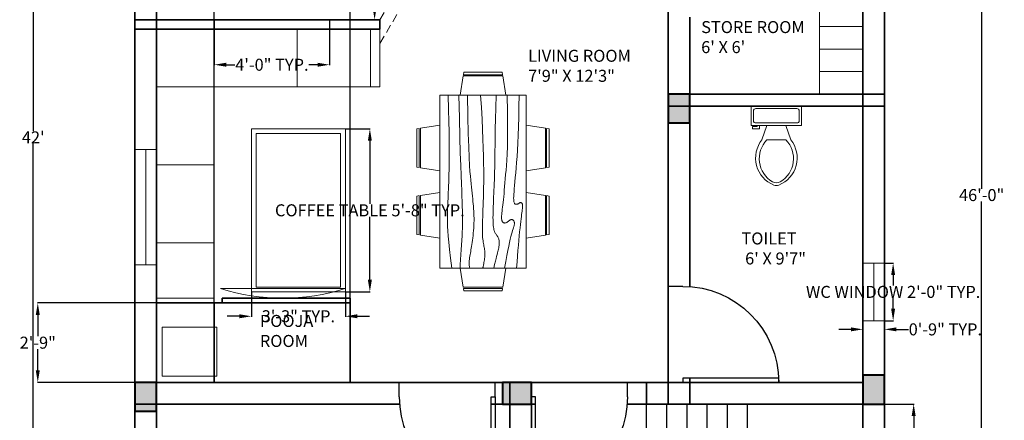
# Model space of a CAD drawing. Units: inches. Extents: x -54 to 881, y -122 to 681.
# Tile 5 of 6: x 472 to 881, y 254 to 421. Entities that reach past the tile are written whole.
import ezdxf

# ---------------------------------------------------------------- set-up
doc = ezdxf.new("R2010")
doc.units = ezdxf.units.IN
doc.header["$MEASUREMENT"] = 0
doc.linetypes.add('DASHED', pattern=[0.75, 0.5, -0.25])
for name, color, linetype, lineweight in [('A-ANNO-DIMS', 2, 'Continuous', 18), ('A-DOOR', 3, 'Continuous', 25), ('A-EQPM', 9, 'Continuous', 18), ('A-FLOR-CASE', 8, 'Continuous', 18), ('A-FLOR-FIXT', 9, 'Continuous', 18), ('A-FLOR-STRS', 7, 'Continuous', 25), ('A-FURN', 8, 'Continuous', 18), ('A-GLAZ', 4, 'Continuous', 20), ('A-WALL', 7, 'Continuous', 35), ('A-WALL-OVHD', 8, 'DASHED', 18)]:
    doc.layers.add(name, color=color, linetype=linetype, lineweight=lineweight)
doc.layers.add('A-AREA-IDEN', color=217, linetype='Continuous', lineweight=18, true_color=0x93278f)
doc.layers.add('A-COLS', color=240, linetype='Continuous', lineweight=40, true_color=0xed1f24)
doc.styles.get("Standard").update_dxf_attribs({"font": 'arial.ttf'})
doc.dimstyles.get("Standard").update_dxf_attribs({"dimtxt": 5, "dimasz": 5, "dimexe": 0.18, "dimexo": 0.0625, "dimgap": 0.09, "dimtad": 0, "dimtih": 1, "dimtoh": 1, "dimdec": 0, "dimzin": 0, "dimdsep": 46, "dimlunit": 3, "dimtxsty": 'Standard', "dimcen": 0.09, "dimadec": 0, "dimazin": 0, "dimtfac": 1, "dimtdec": 0, "dimtofl": 0, "dimtmove": 0, "dimatfit": 3, "dimfxl": 1, "dimtolj": 1, "dimtzin": 0, "dimarcsym": 0})

# ---------------------------------------------------------------- blocks, each defined once
blk = doc.blocks.new('*D14')
at = {"layer": 'A-ANNO-DIMS', "color": 0, "lineweight": -2, "transparency": 16777216}
for p, q in [((519.43, 624), (476.98, 624)), ((477.16, 619), (477.16, 374.6)), ((477.16, 125), (477.16, 369.4)), ((519.43, 120), (476.98, 120))]:
    blk.add_line(p, q, dxfattribs=at)
at = {"layer": 'A-ANNO-DIMS', "color": 0, "transparency": 16777216}
for points in [[(476.32, 619), (477.99, 619), (477.16, 624)], [(476.32, 125), (477.99, 125), (477.16, 120)]]:
    blk.add_solid(points, dxfattribs=at)
at = {"layer": 'Defpoints', "color": 0, "transparency": 16777216}
for p in [(519.49, 624), (477.16, 120), (519.49, 120)]:
    blk.add_point(p, dxfattribs=at)
at = {"layer": 'A-ANNO-DIMS', "color": 0, "transparency": 16777216, "insert": (477.16, 372), "char_height": 5, "attachment_point": 5}
blk.add_mtext("\\A1;42'", dxfattribs=at)
blk = doc.blocks.new('Toilet - top')
for p, q in [((9.5, -6), (9.5, -2)), ((-8, -8.5), (-8, -8)), ((-7, -8), (-7, -9.5)), ((-4, -8), (-6, -14)), ((4, -8), (6, -14)), ((-10, -8.5), (-8, -8.5)), ((-10, -9.5), (-10, -8.5)), ((-7, -9.5), (-10, -9.5)), ((4, -14), (-4, -14))]:
    blk.add_line(p, q)
blk.add_lwpolyline([(10.5, -8), (10.5, 0), (-10.5, 0), (-10.5, -8)], close=True)
for points in [[(-9.5, -2), (-9.5, -6)], [(8.5, -1), (-8.5, -1)], [(-8.5, -7), (8.5, -7)]]:
    blk.add_lwpolyline(points)
for centre, radius, start, end in [((-8.62, -1.88), 0.884, 81.8699, 188.1301), ((8.62, -1.88), 0.884, 351.8699, 98.1301), ((-8.62, -6.12), 0.884, 171.8699, 278.1301), ((8.62, -6.12), 0.884, 261.8699, 8.1301), ((3.52, -21.58), 12.17, 141.4691, 247.9714), ((4.2, -21.82), 11.33, 136.3677, 238.9468), ((-3.52, -21.58), 12.17, 292.0284, 38.5307), ((-4.2, -21.82), 11.33, 301.053, 43.6321), ((0, -27.88), 4, 245.7318, 294.2682), ((0, -29), 4, 254.8605, 285.1395)]:
    blk.add_arc(centre, radius, start, end)
blk = doc.blocks.new('Dining Set - 36 x 72 in.')
for p, q in [((-22.2343, 26.00059), (-23.4847, 17.99762)), ((-22.2304, 26), (-5.7608, 26)), ((-22, 27.5), (-22.1562, 26.50042)), ((-5.8416, 26.5), (-22.1534, 26.5)), ((-22, 27.5), (-6, 27.5)), ((-5.8437, 26.49966), (-6, 27.5)), ((-4.5152, 17.99762), (-5.7655, 25.99926)), ((5.7657, 26.00059), (4.5153, 17.99762)), ((5.7696, 26), (22.2392, 26)), ((6, 27.5), (5.8438, 26.50042)), ((22.1584, 26.5), (5.8466, 26.5)), ((6, 27.5), (22, 27.5)), ((22.1563, 26.49966), (22, 27.5)), ((23.4848, 17.99762), (22.2345, 25.99926)), ((36, 18), (-36, 18)), ((-36, 18), (-36, -18)), ((36, -18), (36, 18)), ((-44.0006, 8.23428), (-35.9976, 9.48474)), ((-44, 8.23041), (-44, -8.23915)), ((44.0006, 8.23428), (35.9976, 9.48474)), ((44, 8.23041), (44, -8.23915)), ((-45.5, 8), (-44.5004, 8.15617)), ((-45.5, 8), (-45.5, -8)), ((-44.5, -8.15843), (-44.5, 8.15338)), ((44.5, -8.15843), (44.5, 8.15338)), ((45.5, 8), (44.5005, 8.15617)), ((45.5, 8), (45.5, -8)), ((-44.4997, -8.15631), (-45.5, -8)), ((44.4997, -8.15631), (45.5, -8)), ((-35.9976, -9.48476), (-43.9993, -8.2345)), ((35.9976, -9.48476), (43.9993, -8.2345)), ((-36, -18), (36, -18)), ((-22.2343, -26.0006), (-23.4847, -17.99762)), ((-4.5152, -17.99762), (-5.7655, -25.99928)), ((5.7657, -26.0006), (4.5153, -17.99762)), ((23.4848, -17.99762), (22.2345, -25.99928)), ((-22.2304, -26), (-5.7608, -26)), ((-22, -27.5), (-22.1562, -26.50044)), ((-5.8416, -26.5), (-22.1534, -26.5)), ((-22, -27.5), (-6, -27.5)), ((-5.8437, -26.49967), (-6, -27.5)), ((5.7696, -26), (22.2392, -26)), ((6, -27.5), (5.8438, -26.50044)), ((22.1584, -26.5), (5.8466, -26.5)), ((6, -27.5), (22, -27.5)), ((22.1563, -26.49967), (22, -27.5))]:
    blk.add_line(p, q)
for points in [[(-36, 15), (-31.1772, 14.97754), (-26.8079, 14.91406), (-22.8538, 14.81543), (-19.276, 14.6875), (-16.0362, 14.53613), (-13.0957, 14.36718), (-10.4159, 14.18652), (-7.9583, 14), (-5.6904, 13.81315), (-3.6035, 13.63021), (-1.6954, 13.45508), (0.0365, 13.29166), (1.5945, 13.14388), (2.9811, 13.01562), (4.1988, 12.9108), (5.25, 12.83333), (6.1393, 12.78613), (6.8802, 12.76823), (7.4883, 12.77767), (7.9792, 12.8125), (8.3685, 12.87077), (8.6719, 12.95052), (8.9049, 13.0498), (9.0833, 13.16666), (9.2205, 13.29899), (9.3216, 13.44401), (9.3895, 13.59879), (9.4271, 13.76041), (9.4373, 13.92594), (9.4232, 14.09245), (9.3875, 14.257), (9.3333, 14.41666), (9.2638, 14.56917), (9.1836, 14.71484), (9.0975, 14.85465), (9.0104, 14.98958), (8.9272, 15.1206), (8.8529, 15.2487), (8.7922, 15.37483), (8.75, 15.5), (8.7305, 15.62467), (8.7344, 15.74739), (8.7617, 15.86621), (8.8125, 15.97916), (8.8867, 16.08431), (8.9844, 16.17968), (9.1055, 16.26334), (9.25, 16.33333), (9.4189, 16.38802), (9.6172, 16.42708), (9.8506, 16.45052), (10.125, 16.45833), (10.4463, 16.45052), (10.8203, 16.42708), (11.2529, 16.38802), (11.75, 16.33333), (12.3184, 16.26318), (12.9694, 16.17838), (13.7151, 16.07991), (14.5677, 15.96875), (15.5395, 15.84586), (16.6426, 15.71224), (17.8893, 15.56884), (19.2917, 15.41666), (20.859, 15.25667), (22.5879, 15.08984), (24.4721, 14.91715), (26.5052, 14.73958), (28.6809, 14.5581), (30.9929, 14.3737), (33.4347, 14.18733), (36, 14)], [(-36, 10), (-28.9766, 10.14274), (-23.1725, 10.20442), (-18.4241, 10.19775), (-14.5677, 10.13541), (-11.4399, 10.03011), (-8.877, 9.89453), (-6.7154, 9.74137), (-4.7917, 9.58333), (-2.9698, 9.43082), (-1.2246, 9.28515), (0.4415, 9.14534), (2.026, 9.01041), (3.5266, 8.87939), (4.9408, 8.7513), (6.266, 8.62516), (7.5, 8.5), (8.6411, 8.37549), (9.6914, 8.2539), (10.6538, 8.13818), (11.5312, 8.03125), (12.3267, 7.93603), (13.043, 7.85547), (13.6831, 7.79248), (14.25, 7.75), (14.7471, 7.7303), (15.1797, 7.73307), (15.5537, 7.75732), (15.875, 7.80208), (16.1494, 7.86637), (16.3828, 7.94922), (16.5811, 8.04964), (16.75, 8.16666), (16.8944, 8.29915), (17.0143, 8.44531), (17.1089, 8.60319), (17.1771, 8.77083), (17.218, 8.94629), (17.2305, 9.1276), (17.2137, 9.31282), (17.1667, 9.5), (17.0895, 9.6875), (16.987, 9.875), (16.8649, 10.0625), (16.7292, 10.25), (16.5856, 10.4375), (16.4401, 10.625), (16.2985, 10.8125), (16.1667, 11), (16.05, 11.18733), (15.9518, 11.3737), (15.8752, 11.5581), (15.8229, 11.73958), (15.798, 11.91715), (15.8034, 12.08984), (15.842, 12.25667), (15.9167, 12.41666), (16.0295, 12.56836), (16.1784, 12.70833), (16.3605, 12.83268), (16.5729, 12.9375), (16.8127, 13.01888), (17.0768, 13.07291), (17.3625, 13.0957), (17.6667, 13.08333), (17.9894, 13.03312), (18.3418, 12.94726), (18.7382, 12.82918), (19.1927, 12.68229), (19.7195, 12.51001), (20.3327, 12.31575), (21.0465, 12.10294), (21.875, 11.875), (22.8357, 11.63354), (23.959, 11.37304), (25.2786, 11.08618), (26.8282, 10.76562), (28.6414, 10.40405), (30.752, 9.99414), (33.1936, 9.52856), (36, 9)], [(-36, 5.5), (-30.7157, 5.3348), (-26.069, 5.20963), (-21.9946, 5.11767), (-18.4271, 5.05208), (-15.3009, 5.00602), (-12.5508, 4.97265), (-10.1112, 4.94515), (-7.9167, 4.91666), (-5.909, 4.88167), (-4.0586, 4.83984), (-2.3429, 4.79215), (-0.7396, 4.73958), (0.7739, 4.6831), (2.22, 4.6237), (3.6213, 4.56233), (5, 4.5), (6.373, 4.43782), (7.7344, 4.3776), (9.0723, 4.32129), (10.375, 4.27083), (11.6309, 4.22819), (12.8281, 4.19531), (13.9551, 4.17415), (15, 4.16666), (15.954, 4.17448), (16.819, 4.19791), (17.6001, 4.23698), (18.3021, 4.29166), (18.9299, 4.36198), (19.4883, 4.44791), (19.9823, 4.54948), (20.4167, 4.66666), (20.7969, 4.79899), (21.1302, 4.94401), (21.4245, 5.09879), (21.6875, 5.26041), (21.9271, 5.42594), (22.1511, 5.59245), (22.3672, 5.757), (22.5834, 5.91666), (22.8065, 6.06868), (23.0404, 6.21093), (23.2879, 6.34147), (23.5521, 6.45833), (23.8358, 6.55957), (24.142, 6.64323), (24.4735, 6.70735), (24.8334, 6.75), (25.2235, 6.76969), (25.642, 6.76692), (26.0858, 6.74267), (26.5521, 6.69791), (27.0379, 6.63362), (27.5404, 6.55078), (28.0565, 6.45036), (28.5834, 6.33333), (29.1242, 6.19987), (29.7071, 6.04687), (30.3661, 5.87044), (31.1354, 5.66666), (32.0493, 5.43164), (33.142, 5.16146), (34.4475, 4.85221), (36, 4.5)], [(-36, -1), (-30.7915, -0.6591), (-26.0195, -0.38216), (-21.6519, -0.16284), (-17.6563, 0.00521), (-14.0005, 0.12833), (-10.6523, 0.21289), (-7.5796, 0.26522), (-4.75, 0.29166), (-2.134, 0.29793), (0.2878, 0.28711), (2.5317, 0.26163), (4.6146, 0.22396), (6.5529, 0.17651), (8.3633, 0.12174), (10.0623, 0.06209), (11.6667, 0), (13.1899, -0.06201), (14.6341, -0.1211), (15.9982, -0.17432), (17.2813, -0.21875), (18.4823, -0.25147), (19.6003, -0.26953), (20.6343, -0.27002), (21.5834, -0.25), (22.4481, -0.20768), (23.2357, -0.14584), (23.9549, -0.06836), (24.6146, 0.02083), (25.2235, 0.11784), (25.7904, 0.21875), (26.3241, 0.31966), (26.8334, 0.41666), (27.3265, 0.50618), (27.8099, 0.58593), (28.2894, 0.65397), (28.7709, 0.70833), (29.2601, 0.74707), (29.763, 0.76823), (30.2855, 0.76985), (30.8334, 0.75), (31.4088, 0.70784), (31.9994, 0.64713), (32.589, 0.57275), (33.1615, 0.48958), (33.7008, 0.4025), (34.1908, 0.3164), (34.6153, 0.23616), (34.9584, 0.16666), (35.2099, 0.11165), (35.3848, 0.07031), (35.504, 0.04069), (35.5886, 0.02083), (35.6594, 0.00879), (35.7377, 0.0026), (35.8442, 0.00032), (36, 0)], [(-36, -6.5), (-27.1843, -6.31267), (-20.084, -6.1263), (-14.469, -5.9419), (-10.1094, -5.76042), (-6.7752, -5.58285), (-4.2363, -5.41016), (-2.2629, -5.24333), (-0.625, -5.08334), (0.8708, -4.93099), (2.2715, -4.78646), (3.5872, -4.64974), (4.8281, -4.52084), (6.0046, -4.39974), (7.127, -4.28646), (8.2053, -4.18099), (9.25, -4.08334), (10.2705, -3.99382), (11.2734, -3.91407), (12.2647, -3.84603), (13.25, -3.79167), (14.2354, -3.75293), (15.2266, -3.73177), (16.2295, -3.73015), (17.25, -3.75), (18.2912, -3.79248), (19.3451, -3.85547), (20.4009, -3.93604), (21.4479, -4.03125), (22.4754, -4.13819), (23.4727, -4.25391), (24.4289, -4.37549), (25.3334, -4.5), (26.1785, -4.62492), (26.9694, -4.74935), (27.7145, -4.87281), (28.4219, -4.99479), (29.1, -5.11483), (29.7572, -5.23242), (30.4016, -5.34709), (31.0417, -5.45834), (31.6837, -5.56437), (32.3262, -5.65821), (32.9658, -5.73153), (33.599, -5.77604), (34.2224, -5.78345), (34.8327, -5.74545), (35.4264, -5.65373), (36, -5.5)], [(-36, -10), (-26.4022, -9.81299), (-18.4675, -9.62891), (-11.9839, -9.45069), (-6.7396, -9.28125), (-2.5226, -9.12354), (0.8789, -8.98047), (3.6769, -8.85498), (6.0833, -8.75), (8.2767, -8.66765), (10.3021, -8.60677), (12.1712, -8.56543), (13.8958, -8.54167), (15.4876, -8.53353), (16.9583, -8.53907), (18.3197, -8.55632), (19.5834, -8.58334), (20.7616, -8.61841), (21.8685, -8.66081), (22.9188, -8.71004), (23.9271, -8.76563), (24.9081, -8.82707), (25.8763, -8.89388), (26.8465, -8.96558), (27.8334, -9.04167), (28.8474, -9.12118), (29.8828, -9.20117), (30.93, -9.27824), (31.9792, -9.34896), (33.0205, -9.40991), (34.0443, -9.45768), (35.0407, -9.48885), (36, -9.5)], [(-36, -14.5), (-30.0881, -14.33513), (-25.0332, -14.21224), (-20.7312, -14.12647), (-17.0781, -14.07292), (-13.97, -14.04671), (-11.3027, -14.04297), (-8.9724, -14.05681), (-6.875, -14.08334), (-4.9224, -14.11833), (-3.0905, -14.16016), (-1.3709, -14.20785), (0.2448, -14.26042), (1.7647, -14.3169), (3.1973, -14.3763), (4.5507, -14.43767), (5.8333, -14.5), (7.0554, -14.5621), (8.235, -14.62175), (9.3922, -14.67652), (10.5469, -14.72396), (11.7192, -14.76164), (12.929, -14.78711), (14.1965, -14.79794), (15.5417, -14.79167), (16.9933, -14.76424), (18.6152, -14.70508), (20.4804, -14.60197), (22.6615, -14.44271), (25.2312, -14.21509), (28.2624, -13.9069), (31.8277, -13.50594), (36, -13)]]:
    blk.add_lwpolyline(points)
blk = doc.blocks.new('*U12')
for p, q in [((0, 0), (0, -6)), ((40, 0), (40, -6))]:
    blk.add_line(p, q)
blk.add_lwpolyline([(0, 0), (0, 40), (1.75, 40), (1.75, 0)], close=True)
blk.add_arc((0, 0), 40, 0, 90)
blk = doc.blocks.new('WIN-48X9')
for p, q in [((0, 0), (0, 9)), ((48, 0), (48, 9)), ((0, 4.5), (48, 4.5))]:
    blk.add_line(p, q)
blk = doc.blocks.new('WIN-24X9')
for p, q in [((0, 24), (9, 24)), ((4.5, 24), (4.5, 0)), ((0, 0), (9, 0))]:
    blk.add_line(p, q)
blk = doc.blocks.new('TV-52-PLAN')
blk.add_line((0, 4), (52, 4))
blk.add_arc((26, 86.41), 86.41, 252.4883, 287.5117)
blk = doc.blocks.new('LIVING-COFFEE-TABLE')
for points in [[(0, 67.86), (39.15, 67.86), (39.15, 0), (0, 0)], [(2, 65.86), (37.15, 65.86), (37.15, 2), (2, 2)]]:
    blk.add_lwpolyline(points, close=True)
blk = doc.blocks.new('STAIR-RETURN-FLIGHT')
for p, q in [((48, 93), (48, 141)), ((56.4, 93), (56.4, 141)), ((64.8, 93), (64.8, 141)), ((73.2, 93), (73.2, 141)), ((81.6, 93), (81.6, 141)), ((90, 93), (90, 141)), ((48, 0), (48, 93)), ((48, 93), (90, 93)), ((48, 91), (90, 91)), ((50, 0), (50, 93)), ((88, 0), (88, 93)), ((90, 0), (90, 93)), ((90, 93), (138, 93)), ((90, 85), (138, 85)), ((90, 77), (138, 77)), ((90, 69), (138, 69)), ((90, 61), (138, 61)), ((0, 57), (48, 57)), ((90, 53), (138, 53)), ((0, 49), (48, 49)), ((0, 41), (48, 41)), ((90, 45), (138, 45)), ((90, 37), (138, 37)), ((0, 33), (48, 33)), ((90, 29), (138, 29)), ((0, 25), (48, 25)), ((90, 21), (138, 21)), ((0, 17), (48, 17)), ((90, 13), (138, 13)), ((0, 9), (48, 9)), ((48, 2), (90, 2)), ((48, 0), (90, 0))]:
    blk.add_line(p, q)
blk = doc.blocks.new('STORAGE-RACK-72X18')
for p, q in [((0, 0), (0, 72)), ((0, 65.625), (18, 65.625)), ((0, 56.25), (18, 56.25)), ((0, 46.875), (18, 46.875)), ((0, 37.5), (18, 37.5)), ((0, 28.125), (18, 28.125)), ((0, 18.75), (18, 18.75)), ((0, 9.375), (18, 9.375)), ((0, 0), (18, 0))]:
    blk.add_line(p, q)
blk = doc.blocks.new('COL-9X12')
h = blk.add_hatch(color=256)
h.dxf.hatch_style = 1
h.paths.add_polyline_path([(9, 12), (0, 12), (0, 0), (9, 0)])
blk.add_lwpolyline([(0, 0), (9, 0), (9, 12), (0, 12)], close=True)
blk = doc.blocks.new('LIVING-SIDE-TABLE')
blk.add_lwpolyline([(0, 20.5), (22.77, 20.5), (22.77, 0), (0, 0)], close=True)
blk = doc.blocks.new('*D44')
at = {"layer": 'A-ANNO-DIMS', "color": 0, "lineweight": -2, "transparency": 16777216}
for p, q in [((831.55, 319.69), (835.27, 319.69)), ((835.09, 314.69), (835.09, 310.36)), ((835.09, 300.69), (835.09, 305.01)), ((831.55, 295.69), (835.27, 295.69))]:
    blk.add_line(p, q, dxfattribs=at)
at = {"layer": 'A-ANNO-DIMS', "color": 0, "transparency": 16777216}
for points in [[(834.26, 314.69), (835.92, 314.69), (835.09, 319.69)], [(834.26, 300.69), (835.92, 300.69), (835.09, 295.69)]]:
    blk.add_solid(points, dxfattribs=at)
at = {"layer": 'Defpoints', "color": 0, "transparency": 16777216}
for p in [(831.49, 319.69), (835.09, 319.69), (831.49, 295.69)]:
    blk.add_point(p, dxfattribs=at)
at = {"layer": 'A-ANNO-DIMS', "color": 0, "transparency": 16777216, "insert": (835.09, 307.69), "char_height": 5, "attachment_point": 5}
blk.add_mtext('\\A1;WC WINDOW 2\'-0" TYP.', dxfattribs=at)
blk = doc.blocks.new('*D45')
at = {"layer": 'A-ANNO-DIMS', "color": 0, "lineweight": -2, "transparency": 16777216}
for p, q in [((822.49, 295.62), (822.49, 291.91)), ((831.49, 295.62), (831.49, 291.91)), ((817.49, 292.09), (812.49, 292.09)), ((836.49, 292.09), (841.49, 292.09))]:
    blk.add_line(p, q, dxfattribs=at)
at = {"layer": 'A-ANNO-DIMS', "color": 0, "transparency": 16777216}
for points in [[(817.49, 292.92), (817.49, 291.25), (822.49, 292.09)], [(836.49, 292.92), (836.49, 291.25), (831.49, 292.09)]]:
    blk.add_solid(points, dxfattribs=at)
at = {"layer": 'Defpoints', "color": 0, "transparency": 16777216}
for p in [(822.49, 295.69), (831.49, 295.69), (831.49, 292.09)]:
    blk.add_point(p, dxfattribs=at)
at = {"layer": 'A-ANNO-DIMS', "color": 0, "transparency": 16777216, "insert": (856.82, 292.09), "char_height": 5, "attachment_point": 5}
blk.add_mtext('\\A1;0\'-9" TYP.', dxfattribs=at)
blk = doc.blocks.new('*D62')
at = {"layer": 'A-ANNO-DIMS', "color": 0, "lineweight": -2, "transparency": 16777216}
for p, q in [((607.15, 375.58), (617.45, 375.58)), ((617.27, 370.58), (617.27, 344.32)), ((617.27, 312.72), (617.27, 338.97)), ((607.15, 307.72), (617.45, 307.72))]:
    blk.add_line(p, q, dxfattribs=at)
at = {"layer": 'A-ANNO-DIMS', "color": 0, "transparency": 16777216}
for points in [[(616.44, 370.58), (618.1, 370.58), (617.27, 375.58)], [(616.44, 312.72), (618.1, 312.72), (617.27, 307.72)]]:
    blk.add_solid(points, dxfattribs=at)
at = {"layer": 'Defpoints', "color": 0, "transparency": 16777216}
for p in [(607.09, 375.58), (617.27, 375.58), (607.09, 307.72)]:
    blk.add_point(p, dxfattribs=at)
at = {"layer": 'A-ANNO-DIMS', "color": 0, "transparency": 16777216, "insert": (617.27, 341.65), "char_height": 5, "attachment_point": 5}
blk.add_mtext('\\A1;COFFEE TABLE 5\'-8" TYP.', dxfattribs=at)
blk = doc.blocks.new('*D63')
at = {"layer": 'A-ANNO-DIMS', "color": 0, "lineweight": -2, "transparency": 16777216}
for p, q in [((567.94, 307.66), (567.94, 297.36)), ((607.09, 307.66), (607.09, 297.36)), ((562.94, 297.54), (557.94, 297.54)), ((612.09, 297.54), (617.09, 297.54))]:
    blk.add_line(p, q, dxfattribs=at)
at = {"layer": 'A-ANNO-DIMS', "color": 0, "transparency": 16777216}
for points in [[(562.94, 298.37), (562.94, 296.71), (567.94, 297.54)], [(612.09, 298.37), (612.09, 296.71), (607.09, 297.54)]]:
    blk.add_solid(points, dxfattribs=at)
at = {"layer": 'Defpoints', "color": 0, "transparency": 16777216}
for p in [(567.94, 307.72), (607.09, 307.72), (607.09, 297.54)]:
    blk.add_point(p, dxfattribs=at)
at = {"layer": 'A-ANNO-DIMS', "color": 0, "transparency": 16777216, "insert": (587.51, 297.54), "char_height": 5, "attachment_point": 5}
blk.add_mtext('\\A1;3\'-3" TYP.', dxfattribs=at)
blk = doc.blocks.new('*D64')
at = {"layer": 'A-ANNO-DIMS', "color": 0, "lineweight": -2, "transparency": 16777216}
for p, q in [((822.55, 261), (843.82, 261)), ((843.64, 256), (843.64, 193.18)), ((843.64, 125), (843.64, 187.82)), ((822.55, 120), (843.82, 120))]:
    blk.add_line(p, q, dxfattribs=at)
at = {"layer": 'A-ANNO-DIMS', "color": 0, "transparency": 16777216}
for points in [[(842.81, 256), (844.47, 256), (843.64, 261)], [(842.81, 125), (844.47, 125), (843.64, 120)]]:
    blk.add_solid(points, dxfattribs=at)
at = {"layer": 'Defpoints', "color": 0, "transparency": 16777216}
for p in [(822.49, 261), (843.64, 261), (822.49, 120)]:
    blk.add_point(p, dxfattribs=at)
at = {"layer": 'A-ANNO-DIMS', "color": 0, "transparency": 16777216, "insert": (843.64, 190.5), "char_height": 5, "attachment_point": 5}
blk.add_mtext('\\A1;STAIR 11\'-9" TYP.', dxfattribs=at)
blk = doc.blocks.new('*D66')
at = {"layer": 'A-ANNO-DIMS', "color": 0, "lineweight": -2, "transparency": 16777216}
for p, q in [((600.55, 546), (619.42, 546)), ((619.24, 541), (619.24, 486.18)), ((619.24, 426), (619.24, 480.82)), ((600.55, 421), (619.42, 421))]:
    blk.add_line(p, q, dxfattribs=at)
at = {"layer": 'A-ANNO-DIMS', "color": 0, "transparency": 16777216}
for points in [[(618.41, 541), (620.07, 541), (619.24, 546)], [(618.41, 426), (620.07, 426), (619.24, 421)]]:
    blk.add_solid(points, dxfattribs=at)
at = {"layer": 'Defpoints', "color": 0, "transparency": 16777216}
for p in [(600.49, 546), (619.24, 546), (600.49, 421)]:
    blk.add_point(p, dxfattribs=at)
at = {"layer": 'A-ANNO-DIMS', "color": 0, "transparency": 16777216, "insert": (619.24, 483.5), "char_height": 5, "attachment_point": 5}
blk.add_mtext('\\A1;COUNTER 10\'-5" TYP.', dxfattribs=at)
blk = doc.blocks.new('*D67')
at = {"layer": 'A-ANNO-DIMS', "color": 0, "lineweight": -2, "transparency": 16777216}
for p, q in [((552.49, 420.94), (552.49, 402.07)), ((600.49, 420.94), (600.49, 402.07)), ((557.49, 402.25), (561.06, 402.25)), ((595.49, 402.25), (591.92, 402.25))]:
    blk.add_line(p, q, dxfattribs=at)
at = {"layer": 'A-ANNO-DIMS', "color": 0, "transparency": 16777216}
for points in [[(557.49, 403.08), (557.49, 401.42), (552.49, 402.25)], [(595.49, 403.08), (595.49, 401.42), (600.49, 402.25)]]:
    blk.add_solid(points, dxfattribs=at)
at = {"layer": 'Defpoints', "color": 0, "transparency": 16777216}
for p in [(552.49, 421), (600.49, 421), (600.49, 402.25)]:
    blk.add_point(p, dxfattribs=at)
at = {"layer": 'A-ANNO-DIMS', "color": 0, "transparency": 16777216, "insert": (576.49, 402.25), "char_height": 5, "attachment_point": 5}
blk.add_mtext('\\A1;4\'-0" TYP.', dxfattribs=at)
blk = doc.blocks.new('*D75')
at = {"layer": 'A-ANNO-DIMS', "color": 0, "lineweight": -2, "transparency": 16777216}
for p, q in [((831.55, 624), (872.12, 624)), ((871.94, 619), (871.94, 350.64)), ((871.94, 77), (871.94, 345.36)), ((831.55, 72), (872.12, 72))]:
    blk.add_line(p, q, dxfattribs=at)
at = {"layer": 'A-ANNO-DIMS', "color": 0, "transparency": 16777216}
for points in [[(871.11, 619), (872.77, 619), (871.94, 624)], [(871.11, 77), (872.77, 77), (871.94, 72)]]:
    blk.add_solid(points, dxfattribs=at)
at = {"layer": 'Defpoints', "color": 0, "transparency": 16777216}
for p in [(831.49, 624), (871.94, 624), (831.49, 72)]:
    blk.add_point(p, dxfattribs=at)
at = {"layer": 'A-ANNO-DIMS', "color": 0, "transparency": 16777216, "insert": (871.94, 348), "char_height": 5, "attachment_point": 5}
blk.add_mtext('\\A1;46\'-0"', dxfattribs=at)
blk = doc.blocks.new('*D78')
at = {"layer": 'A-ANNO-DIMS', "color": 0, "lineweight": -2, "transparency": 16777216}
for p, q in [((552.43, 303.1), (478.86, 303.1)), ((479.04, 298.1), (479.04, 289.19)), ((479.04, 275), (479.04, 283.91)), ((552.43, 270), (478.86, 270))]:
    blk.add_line(p, q, dxfattribs=at)
at = {"layer": 'A-ANNO-DIMS', "color": 0, "transparency": 16777216}
for points in [[(478.21, 298.1), (479.87, 298.1), (479.04, 303.1)], [(478.21, 275), (479.87, 275), (479.04, 270)]]:
    blk.add_solid(points, dxfattribs=at)
at = {"layer": 'Defpoints', "color": 0, "transparency": 16777216}
for p in [(479.04, 303.1), (552.49, 303.1), (552.49, 270)]:
    blk.add_point(p, dxfattribs=at)
at = {"layer": 'A-ANNO-DIMS', "color": 0, "transparency": 16777216, "insert": (479.04, 286.55), "char_height": 5, "attachment_point": 5}
blk.add_mtext('\\A1;2\'-9"', dxfattribs=at)
blk = doc.blocks.new('*D79')
at = {"layer": 'A-ANNO-DIMS', "color": 0, "lineweight": -2, "transparency": 16777216}
for p, q in [((552.49, 270.06), (552.49, 664.63)), ((557.49, 664.45), (568.12, 664.45)), ((604.07, 664.45), (593.44, 664.45)), ((609.07, 270.06), (609.07, 664.63))]:
    blk.add_line(p, q, dxfattribs=at)
at = {"layer": 'A-ANNO-DIMS', "color": 0, "transparency": 16777216}
for points in [[(557.49, 665.28), (557.49, 663.62), (552.49, 664.45)], [(604.07, 665.28), (604.07, 663.62), (609.07, 664.45)]]:
    blk.add_solid(points, dxfattribs=at)
at = {"layer": 'Defpoints', "color": 0, "transparency": 16777216}
for p in [(609.07, 664.45), (552.49, 270), (609.07, 270)]:
    blk.add_point(p, dxfattribs=at)
at = {"layer": 'A-ANNO-DIMS', "color": 0, "transparency": 16777216, "insert": (580.78, 664.45), "char_height": 5, "attachment_point": 5}
blk.add_mtext('\\A1;4\'-8 1/2"', dxfattribs=at)

msp = doc.modelspace()

# ---------------------------------------------------------------- linework, layer by layer
at = {"layer": 'A-FURN'}
for p, q in [((552.49, 305.1), (552.49, 421)), ((552.49, 417), (621.49, 417)), ((586.99, 417), (586.99, 393)), ((617.49, 393), (617.49, 417)), ((621.49, 393), (621.49, 417)), ((528.49, 393), (552.49, 393)), ((552.49, 393), (621.49, 393)), ((528.49, 360.55), (552.49, 360.55)), ((528.49, 328.1), (552.49, 328.1)), ((528.49, 305.1), (552.49, 305.1))]:
    msp.add_line(p, q, dxfattribs=at)
at = {"layer": 'A-WALL'}
for p, q in [((519.49, 72), (519.49, 624)), ((831.49, 120), (831.49, 624)), ((528.49, 421), (528.49, 546)), ((741.49, 261), (741.49, 462)), ((822.49, 390), (822.49, 462)), ((519.49, 421), (621.49, 421)), ((528.49, 270), (528.49, 421)), ((621.49, 421), (621.49, 417)), ((750.49, 309.89), (750.49, 422.11)), ((519.49, 417), (621.49, 417)), ((741.49, 390), (831.49, 390)), ((822.49, 120), (822.49, 390)), ((741.49, 385), (831.49, 385)), ((555.83, 305.1), (609.07, 305.1)), ((555.83, 305.1), (555.83, 303.1)), ((609.07, 305.1), (609.07, 270)), ((528.49, 303.1), (552.49, 303.1)), ((552.49, 270), (552.49, 303.1)), ((552.49, 303.1), (609.07, 303.1)), ((750.49, 261), (750.49, 271.75)), ((519.49, 270), (822.49, 270)), ((528.49, 120), (528.49, 270)), ((675.49, 120), (675.49, 270)), ((684.49, 120), (684.49, 270)), ((732.49, 261), (732.49, 270)), ((519.49, 261), (629.6, 261)), ((667.74, 261), (686.24, 261)), ((724.38, 261), (822.49, 261))]:
    msp.add_line(p, q, dxfattribs=at)
at = {"layer": 'A-WALL-OVHD', "ltscale": 7}
for p, q in [((621.49, 421), (645.49, 462)), ((621.49, 411.1), (651.28, 462))]:
    msp.add_line(p, q, dxfattribs=at)

# ---------------------------------------------------------------- block references
at = {"layer": 'A-COLS'}
for p in [(741.49, 378), (822.49, 261), (519.49, 258)]:
    msp.add_blockref('COL-9X12', p, dxfattribs=at)
at = {"layer": 'A-COLS', "rotation": 90.00000000000048}
msp.add_blockref('COL-9X12', (684.49, 261), dxfattribs=at)
at = {"layer": 'A-DOOR', "xscale": -1}
for p, rotation in [((747.49, 270), 270), ((684.49, 264), 180)]:
    msp.add_blockref('*U12', p, dxfattribs=dict(at, rotation=rotation))
at = {"layer": 'A-DOOR', "rotation": 180}
msp.add_blockref('*U12', (669.49, 264), dxfattribs=at)
at = {"layer": 'A-EQPM'}
msp.add_blockref('TV-52-PLAN', (555.04, 305.1), dxfattribs=at)
at = {"layer": 'A-FLOR-CASE'}
msp.add_blockref('STORAGE-RACK-72X18', (804.49, 390), dxfattribs=at)
at = {"layer": 'A-FLOR-FIXT'}
msp.add_blockref('Toilet - top', (786.49, 385), dxfattribs=at)
at = {"layer": 'A-FLOR-STRS'}
msp.add_blockref('STAIR-RETURN-FLIGHT', (684.49, 120), dxfattribs=at)
at = {"layer": 'A-FURN', "rotation": 270}
msp.add_blockref('Dining Set - 36 x 72 in.', (664.36, 353.59), dxfattribs=at)
at = {"layer": 'A-FURN'}
for name, p in [('LIVING-COFFEE-TABLE', (567.94, 307.72)), ('LIVING-SIDE-TABLE', (530.85, 272.54))]:
    msp.add_blockref(name, p, dxfattribs=at)
at = {"layer": 'A-GLAZ', "rotation": 90}
msp.add_blockref('WIN-48X9', (528.49, 318.95), dxfattribs=at)
at = {"layer": 'A-GLAZ'}
msp.add_blockref('WIN-24X9', (822.49, 295.69), dxfattribs=at)

# ---------------------------------------------------------------- texts
at = {"layer": 'A-AREA-IDEN', "char_height": 5, "attachment_point": 1}
for s, insert in [("STORE ROOM\\P6' X 6'", (755.19, 420.42)), ('LIVING ROOM\\P7\'9" X 12\'3"', (683.13, 408.47)), ('TOILET\\P 6\' X 9\'7"', (771.95, 332.43)), ('POOJA \\PROOM', (571.49, 298.1))]:
    msp.add_mtext_dynamic_manual_height_columns(s, width=65.2326, gutter_width=1, heights=[0], dxfattribs=dict(at, insert=insert))

# ---------------------------------------------------------------- dimensions: what is measured, and where the dimension line sits
at = {"layer": 'A-ANNO-DIMS'}
dim = msp.add_linear_dim(base=(609.07, 664.45), p1=(552.49, 270), p2=(609.07, 270), dimstyle='Standard', override={"dimdec": 1, "dimlfac": 1, "dimrnd": 0, "dimzin": 1, "dimdsep": 46, "dimlunit": 4, "dimfrac": 2}, dxfattribs=at)
dim.commit()
dim.dimension.update_dxf_attribs({"geometry": '*D79', "text_midpoint": (580.78, 664.45)})
for base, p1, p2, override, picture, middle in [((477.16, 120), (519.49, 624), (519.49, 120), {"dimclrd": 0, "dimclre": 0, "dimclrt": 0}, '*D14', (477.16, 372)), ((871.94, 624), (831.49, 72), (831.49, 624), {"dimdec": 1, "dimlfac": 1, "dimrnd": 0, "dimzin": 1, "dimdsep": 46, "dimlunit": 4, "dimfrac": 2}, '*D75', (871.94, 348)), ((479.04, 303.1), (552.49, 270), (552.49, 303.1), {"dimdec": 1, "dimlfac": 1, "dimrnd": 0, "dimzin": 1, "dimdsep": 46, "dimlunit": 4, "dimfrac": 2}, '*D78', (479.04, 286.55))]:
    dim = msp.add_linear_dim(base=base, p1=p1, p2=p2, angle=90, dimstyle='Standard', override=override, dxfattribs=at)
    dim.commit()
    dim.dimension.update_dxf_attribs({"geometry": picture, "text_midpoint": middle})
for base, p1, p2, text, picture, middle in [((619.24, 546), (600.49, 421), (600.49, 546), 'COUNTER <> TYP.', '*D66', (619.24, 483.5)), ((617.27, 375.58), (607.09, 307.72), (607.09, 375.58), 'COFFEE TABLE <> TYP.', '*D62', (617.27, 341.65)), ((835.09, 319.69), (831.49, 295.69), (831.49, 319.69), 'WC WINDOW <> TYP.', '*D44', (835.09, 307.69)), ((843.64, 261), (822.49, 120), (822.49, 261), 'STAIR <> TYP.', '*D64', (843.64, 190.5))]:
    dim = msp.add_linear_dim(base=base, p1=p1, p2=p2, angle=90, text=text, dimstyle='Standard', override={"dimdec": 1, "dimlfac": 1, "dimrnd": 0, "dimzin": 1, "dimdsep": 46, "dimlunit": 4, "dimfrac": 2}, dxfattribs=at)
    dim.commit()
    dim.dimension.update_dxf_attribs({"geometry": picture, "text_midpoint": middle})
for base, p1, p2, picture, middle in [((600.49, 402.25), (552.49, 421), (600.49, 421), '*D67', (576.49, 402.25)), ((607.0909, 297.5409), (567.9365, 307.7193), (607.0909, 307.7193), '*D63', (587.5137, 297.5409)), ((831.49, 292.09), (822.49, 295.69), (831.49, 295.69), '*D45', (856.82, 292.09))]:
    dim = msp.add_linear_dim(base=base, p1=p1, p2=p2, text='<> TYP.', dimstyle='Standard', override={"dimdec": 1, "dimlfac": 1, "dimrnd": 0, "dimzin": 1, "dimdsep": 46, "dimlunit": 4, "dimfrac": 2}, dxfattribs=at)
    dim.commit()
    dim.dimension.update_dxf_attribs({"geometry": picture, "text_midpoint": middle})

doc.saveas('drawing.dxf')
